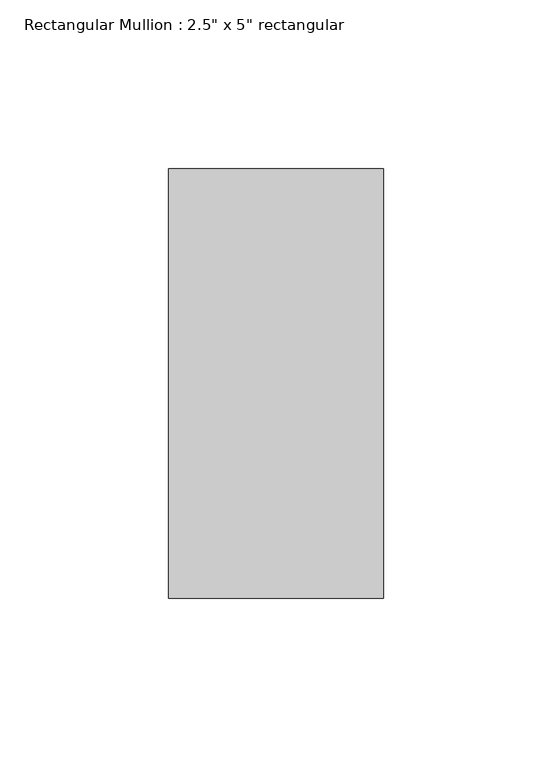
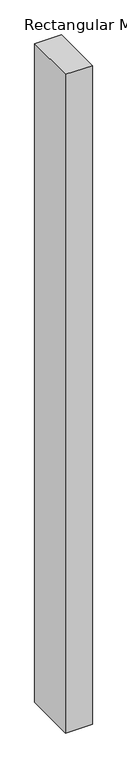
"""IFC4 building model written with IfcOpenShell, lengths in millimetres: member geometry."""

from ifc_helpers import new_model, si_unit, frame, origin, place, context, project, spatial, polyline, outline, extrude, source, transform, mapped, element, save


def member_8ed2a5b7(model_context):
    return source(origin(), model_context, "Body", "SweptSolid", [
        extrude(outline(polyline([(0.0, 63.5), (0.0, -63.5), (-63.5, -63.5), (-63.5, 63.5), (0.0, 63.5)])), frame((0.0, 0.0, -1653.9366569), z_axis=(0.0, 0.0, 1.0), x_axis=(1.0, 0.0, 0.0)), (0.0, 0.0, 1.0), 1653.9366569),
    ])


if __name__ == "__main__":
    model = new_model("IFC4")
    model_context = context("Model", 3, world=origin())
    ifc_project = project(units=[si_unit("LENGTHUNIT", "METRE", prefix="MILLI")], contexts=[model_context])
    site = spatial("IfcSite", under=ifc_project)
    building = spatial("IfcBuilding", under=site)
    placement = place(None, origin())
    member_shape = member_8ed2a5b7(model_context)
    element("IfcMember", 1, ObjectType="Rectangular Mullion : 2.5\" x 5\" rectangular", at=placement, inside=building, context=model_context, shape_type="MappedRepresentation", body=[
        mapped(member_shape, transform((0.0, 0.0, 0.0), x_axis=(1.0, 0.0, 0.0), y_axis=(0.0, 1.0, 0.0), z_axis=(0.0, 0.0, 1.0))),
    ])
    save(model, "model.ifc")

# Revit data of these elements
# Type "Rectangular Mullion : 2.5\" x 5\" rectangular"
#   built-in parameter 1007304 = 0.416667 (stored number, unit not read)
#   built-in parameter 1007301 = 0.104167 (stored number, unit not read)
#   built-in parameter 1007300 = 0.104167 (stored number, unit not read)
# Element 1 (IfcMember, "Rectangular Mullion : 2.5\" x 5\" rectangular")
#   Materials on its faces: "Aluminum"
# Materials
#   "Aluminum": class "Metal", colour RGB 247 247 247, transparency 0, Description = "Aluminum 6061", Cost = 0
